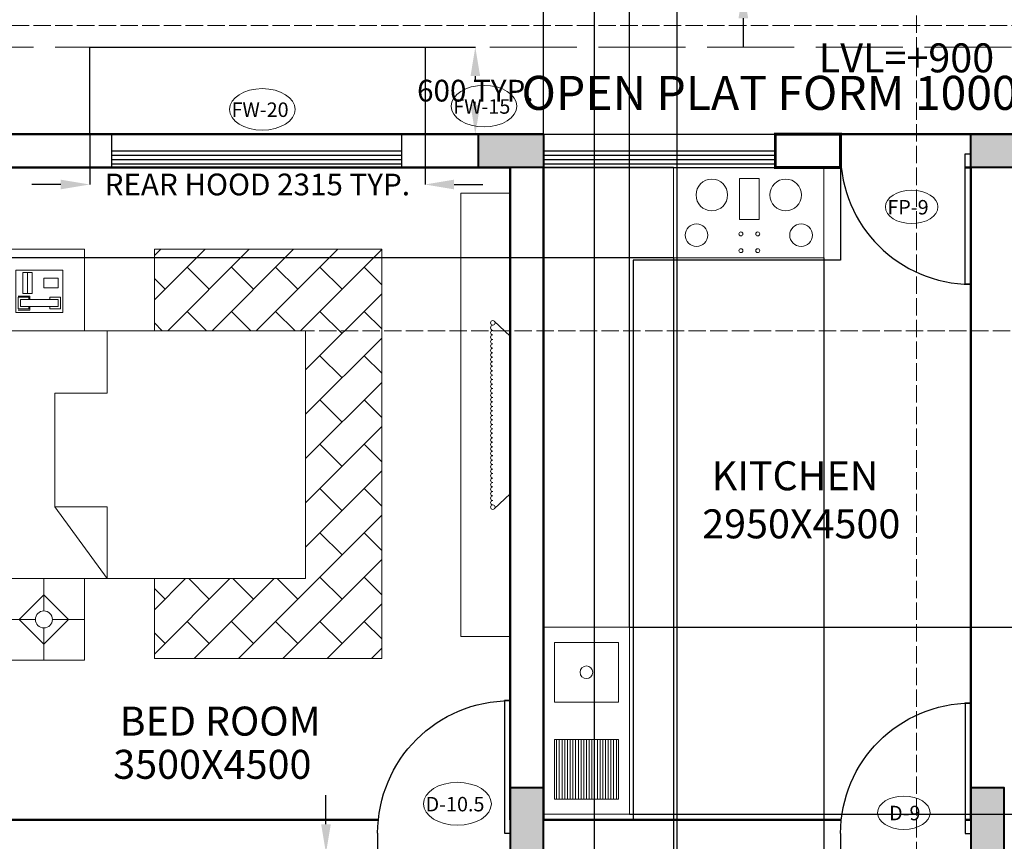
# Model space of a CAD drawing. Units: inches. Extents: x 22626 to 57351, y 2118 to 36234.
# Tile 5 of 10: x 34432 to 41227, y 23379 to 29046. Entities that reach past the tile are written whole.
import ezdxf

# ---------------------------------------------------------------- set-up
doc = ezdxf.new("R2010")
doc.units = ezdxf.units.IN
doc.header["$MEASUREMENT"] = 0
doc.linetypes.add('ACAD_ISO02W100', pattern=[15, 12, -3])
for name, color, linetype, lineweight in [('A-ANNO-DIMS', 130, 'Continuous', 18), ('A-ANNO-IDEN', 130, 'Continuous', 15), ('A-ANNO-SYMB', 130, 'Continuous', 18), ('A-AREA-IDEN', 130, 'Continuous', 18), ('A-COLS', 7, 'Continuous', 40), ('A-EQPM', 30, 'Continuous', 18), ('A-FIXT-PATT', 8, 'Continuous', 13), ('A-FLOR-CASE', 30, 'Continuous', 25), ('A-FLOR-FIXT', 30, 'Continuous', 18), ('A-ROOF', 80, 'Continuous', 25), ('A-ROOF-OVHD', 80, 'ACAD_ISO02W100', 18), ('A-WALL', 80, 'Continuous', 50), ('DOORS', 32, 'Continuous', 25), ('FURNITURE', 30, 'Continuous', 18), ('WINDOWS', 212, 'Continuous', 25)]:
    doc.layers.add(name, color=color, linetype=linetype, lineweight=lineweight)
doc.layers.add('A-SECT', color=2, linetype='ACAD_ISO02W100', lineweight=18, true_color=0xf1eb1f)
doc.styles.get("Standard").update_dxf_attribs({"font": 'arial.ttf'})
doc.dimstyles.get("Standard").update_dxf_attribs({"dimtxt": 150, "dimasz": 200, "dimexe": 0.18, "dimexo": 0.0625, "dimgap": 0.09, "dimtad": 0, "dimtih": 1, "dimtoh": 1, "dimdec": 0, "dimzin": 0, "dimdsep": 46, "dimtxsty": 'Standard', "dimcen": 0.09, "dimadec": 0, "dimazin": 0, "dimtfac": 1, "dimtdec": 0, "dimtofl": 0, "dimtmove": 0, "dimatfit": 3, "dimfxl": 1, "dimtolj": 1, "dimtzin": 0, "dimarcsym": 0})

# ---------------------------------------------------------------- blocks, each defined once
blk = doc.blocks.new('*U7')
for p, q in [((0, 0), (0, -6)), ((40, 0), (40, -6))]:
    blk.add_line(p, q)
blk.add_lwpolyline([(0, 0), (0, 40), (1.75, 40), (1.75, 0)], close=True)
blk.add_arc((0, 0), 40, 0, 90)
blk = doc.blocks.new('Phone - Desk')
for p, q in [((-4.5, -5), (-4.5, 5)), ((-4.5, 5), (4.5, 5)), ((-4, 4.5), (-4, 2)), ((-3.75, 4.5), (-3.75, 2.25)), ((-1.25, 4.5), (-3.75, 4.5)), ((-1.25, 2.25), (-1.25, 4.5)), ((-1, 2), (-1, 4.5)), ((4.5, 5), (4.5, -5)), ((-3.75, 2.25), (-3.25, 2.25)), ((-3.25, 4), (-3.25, -4)), ((-3.25, 4), (-1.75, 4)), ((-1.75, -4), (-1.75, 4)), ((-1.75, 2.25), (-1.25, 2.25)), ((4, 3.5), (-0.5, 3.5)), ((-0.5, 3.5), (-0.5, 1.5)), ((-0.5, 2.5), (4, 2.5)), ((4, 1.5), (4, 3.5)), ((-4, 2), (-3.25, 2)), ((-1.75, 2), (-1, 2)), ((-0.5, 1.5), (4, 1.5)), ((2.75, -1), (0.75, -1)), ((0.75, -1), (0.75, -4)), ((2.75, -4), (2.75, -1)), ((-3.75, -2.25), (-3.25, -2.25)), ((-3.75, -4.5), (-3.75, -2.25)), ((-3.25, -4), (-1.75, -4)), ((-1.75, -2.25), (-1.25, -2.25)), ((-1.25, -2.25), (-1.25, -4.5)), ((0.75, -4), (2.75, -4)), ((4.5, -5), (-4.5, -5)), ((-1.25, -4.5), (-3.75, -4.5))]:
    blk.add_line(p, q)
blk = doc.blocks.new('BED')
h = blk.add_hatch()
h.set_pattern_fill('AR-B816', color=256, scale=27, angle=45)
h.paths.add_polyline_path([(36405.4, 26900.7), (36405.4, 25190.7), (35361.4, 25190.7), (35361.4, 24640.2), (36930.7, 24640.2), (36930.7, 25190.7), (36930.7, 27463.4), (36405.4, 27463.4), (35361.4, 27463.4), (35361.4, 26900.7)])
for p, q in [((35361.4, 26900.7), (35361.4, 27463.4)), ((35361.4, 27463.4), (36405.4, 27463.4)), ((36405.4, 27463.4), (36930.7, 27463.4)), ((36930.7, 27463.4), (36930.7, 25190.7)), ((35034.9, 26900.7), (35034.9, 26469.4)), ((34673.2, 25686.3), (34673.2, 26469.4)), ((35034.9, 26469.4), (34673.2, 26469.4)), ((35034.9, 25686.3), (34673.2, 25686.3)), ((34673.2, 25686.3), (35034.9, 25190.7)), ((35034.9, 25190.7), (35034.9, 25686.3)), ((34598.8, 25190.7), (34598.8, 24968.4)), ((35361.4, 24640.2), (35361.4, 25190.7)), ((36930.7, 25190.7), (36930.7, 24640.2)), ((34428.6, 24909.4), (34598.8, 25079.6)), ((34598.8, 25079.6), (34768.9, 24909.4)), ((34317.4, 24909.4), (34539.7, 24909.4)), ((34598.8, 24739.2), (34428.6, 24909.4)), ((34768.9, 24909.4), (34598.8, 24739.2)), ((34657.8, 24909.4), (34880.1, 24909.4)), ((34598.8, 24850.4), (34598.8, 24628.1)), ((36930.7, 24640.2), (35361.4, 24640.2))]:
    blk.add_line(p, q)
for points in [[(34317.4, 26900.7), (34880.1, 26900.7), (34880.1, 27463.4), (34317.4, 27463.4)], [(34317.4, 26900.7), (36405.4, 26900.7), (36405.4, 25190.7), (34317.4, 25190.7)], [(34317.4, 25190.7), (34880.1, 25190.7), (34880.1, 24628.1), (34317.4, 24628.1)]]:
    blk.add_lwpolyline(points, close=True)
blk.add_circle((34598.8, 24909.4), 59)
at = {"xscale": 32.52267765020765, "yscale": 32.52267765020765, "zscale": 32.52267765020765, "rotation": 90}
blk.add_blockref('Phone - Desk', (34567, 27172.9), dxfattribs=at)
blk = doc.blocks.new('*D20')
at = {"layer": 'A-ANNO-DIMS', "color": 0, "lineweight": -2, "transparency": 16777216}
for p, q in [((39426.2, 29756.9), (39426.2, 29956.9)), ((40218, 29556.9), (39426, 29556.9)), ((40218, 29256.9), (39426, 29256.9)), ((39426.2, 29056.9), (39426.2, 28856.9))]:
    blk.add_line(p, q, dxfattribs=at)
at = {"layer": 'A-ANNO-DIMS', "color": 0, "transparency": 16777216}
for points in [[(39392.9, 29756.9), (39459.5, 29756.9), (39426.2, 29556.9)], [(39392.9, 29056.9), (39459.5, 29056.9), (39426.2, 29256.9)]]:
    blk.add_solid(points, dxfattribs=at)
at = {"layer": 'Defpoints', "color": 0, "transparency": 16777216}
for p in [(39426.2, 29556.9), (40218, 29556.9), (40218, 29256.9)]:
    blk.add_point(p, dxfattribs=at)
at = {"layer": 'A-ANNO-DIMS', "color": 0, "transparency": 16777216, "insert": (39426.2, 29406.9), "char_height": 150, "attachment_point": 5}
blk.add_mtext('\\A1;300', dxfattribs=at)
blk = doc.blocks.new('BEDROOM-WALL-UNIT-LARGE')
for p, q in [((340.4, 2073.4), (230, 2176.6)), ((340.4, 2073.4), (340.4, 984.3)), ((340.4, 984.3), (230, 881.1))]:
    blk.add_line(p, q)
blk.add_lwpolyline([(340.4, 3057.7), (0, 3057.7), (0, 0), (340.4, 0)], close=True)
for centre in [(220.4, 2164.5), (220.4, 893.2)]:
    blk.add_circle(centre, 15.4)
for centre, radius, start, end in [((223.5, 2130.6), 18.8, 99.47834, 260.52166), ((220.4, 2096.6), 15.4, 90, 270), ((220.4, 2065.7), 15.4, 90, 270), ((220.4, 2034.9), 15.4, 90, 270), ((220.4, 2004), 15.4, 90, 270), ((220.4, 1973.2), 15.4, 90, 270), ((220.4, 1942.3), 15.4, 90, 270), ((220.4, 1911.5), 15.4, 90, 270), ((220.4, 1880.6), 15.4, 90, 270), ((220.4, 1849.7), 15.4, 90, 270), ((220.4, 1818.9), 15.4, 90, 270), ((220.4, 1788), 15.4, 90, 270), ((220.4, 1757.2), 15.4, 90, 270), ((220.4, 1726.3), 15.4, 90, 270), ((220.4, 1695.5), 15.4, 90, 270), ((220.4, 1664.6), 15.4, 90, 270), ((220.4, 1633.8), 15.4, 90, 270), ((220.4, 1602.9), 15.4, 90, 270), ((220.4, 1572), 15.4, 90, 270), ((220.4, 1541.2), 15.4, 90, 270), ((220.4, 1510.3), 15.4, 90, 270), ((220.4, 1479.5), 15.4, 90, 270), ((220.4, 1448.6), 15.4, 90, 270), ((220.4, 1417.8), 15.4, 90, 270), ((220.4, 1386.9), 15.4, 90, 270), ((220.4, 1356), 15.4, 90, 270), ((220.4, 1325.2), 15.4, 90, 270), ((220.4, 1294.3), 15.4, 90, 270), ((220.4, 1263.5), 15.4, 90, 270), ((220.4, 1232.6), 15.4, 90, 270), ((220.4, 1201.8), 15.4, 90, 270), ((220.4, 1170.9), 15.4, 90, 270), ((220.4, 1140), 15.4, 90, 270), ((220.4, 1109.2), 15.4, 90, 270), ((220.4, 1078.3), 15.4, 90, 270), ((220.4, 1047.5), 15.4, 90, 270), ((220.4, 1016.6), 15.4, 90, 270), ((220.4, 985.8), 15.4, 90, 270), ((220.4, 954.9), 15.4, 90, 270), ((220.4, 924), 15.4, 90, 270)]:
    blk.add_arc(centre, radius, start, end)
blk = doc.blocks.new('WIN-FIXED-2000-REAR')
for p, q in [((0, 114.3), (2000, 114.3)), ((0, 84.3), (2000, 84.3)), ((0, 54.3), (2000, 54.3)), ((0, 24.3), (2000, 24.3))]:
    blk.add_line(p, q)
blk.add_lwpolyline([(0, 230), (2000, 230), (2000, 0), (0, 0), (0, 230)])
blk = doc.blocks.new('COL-RECTANGULAR')
h = blk.add_hatch(color=256)
h.dxf.hatch_style = 1
h.paths.add_polyline_path([(0, 0), (450, 0), (450, 230), (0, 230)])
blk.add_lwpolyline([(0, 0), (0, 230), (450, 230), (450, 0)], close=True)
blk = doc.blocks.new('WINDOW-HOOD')
for p, q in [((0, 0), (0, 600)), ((0, 600), (2314.6, 600)), ((2314.6, 600), (2314.6, 0))]:
    blk.add_line(p, q)
blk = doc.blocks.new('*D53')
at = {"layer": 'A-ANNO-DIMS', "color": 0, "lineweight": -2, "transparency": 16777216}
for p, q in [((36545.6, 23496.9), (36545.6, 23696.9)), ((36412.5, 23296.9), (36545.7, 23296.9)), ((36412.5, 22941.5), (36545.7, 22941.5)), ((36545.6, 22741.5), (36545.6, 22541.5))]:
    blk.add_line(p, q, dxfattribs=at)
at = {"layer": 'A-ANNO-DIMS', "color": 0, "transparency": 16777216}
for points in [[(36512.2, 23496.9), (36578.9, 23496.9), (36545.6, 23296.9)], [(36512.2, 22741.5), (36578.9, 22741.5), (36545.6, 22941.5)]]:
    blk.add_solid(points, dxfattribs=at)
at = {"layer": 'Defpoints', "color": 0, "transparency": 16777216}
for p in [(36412.4, 23296.9), (36545.6, 23296.9), (36412.4, 22941.5)]:
    blk.add_point(p, dxfattribs=at)
at = {"layer": 'A-ANNO-DIMS', "color": 0, "transparency": 16777216, "insert": (36545.6, 23119.2), "char_height": 150, "attachment_point": 5}
blk.add_mtext('\\A1;355 TYP.', dxfattribs=at)
blk = doc.blocks.new('*D86')
at = {"layer": 'A-ANNO-DIMS', "color": 0, "lineweight": -2, "transparency": 16777216}
for p, q in [((34914.8, 28256.8), (34914.8, 27909.5)), ((37229.4, 28256.8), (37229.4, 27909.5)), ((34714.8, 27909.7), (34514.8, 27909.7)), ((37429.4, 27909.7), (37629.4, 27909.7))]:
    blk.add_line(p, q, dxfattribs=at)
at = {"layer": 'A-ANNO-DIMS', "color": 0, "transparency": 16777216}
for points in [[(34714.8, 27943), (34714.8, 27876.3), (34914.8, 27909.7)], [(37429.4, 27943), (37429.4, 27876.3), (37229.4, 27909.7)]]:
    blk.add_solid(points, dxfattribs=at)
at = {"layer": 'Defpoints', "color": 0, "transparency": 16777216}
for p in [(34914.8, 28256.9), (37229.4, 28256.9), (37229.4, 27909.7)]:
    blk.add_point(p, dxfattribs=at)
at = {"layer": 'A-ANNO-DIMS', "color": 0, "transparency": 16777216, "insert": (36072.1, 27909.7), "char_height": 150, "attachment_point": 5}
blk.add_mtext('\\A1;REAR HOOD 2315 TYP.', dxfattribs=at)
blk = doc.blocks.new('*D87')
at = {"layer": 'A-ANNO-DIMS', "color": 0, "lineweight": -2, "transparency": 16777216}
for p, q in [((37229.4, 28856.9), (37576.7, 28856.9)), ((37576.5, 28656.9), (37576.5, 28633.5)), ((37576.5, 28456.9), (37576.5, 28480.2)), ((37229.4, 28256.9), (37576.7, 28256.9))]:
    blk.add_line(p, q, dxfattribs=at)
at = {"layer": 'A-ANNO-DIMS', "color": 0, "transparency": 16777216}
for points in [[(37543.2, 28656.9), (37609.9, 28656.9), (37576.5, 28856.9)], [(37543.2, 28456.9), (37609.9, 28456.9), (37576.5, 28256.9)]]:
    blk.add_solid(points, dxfattribs=at)
at = {"layer": 'Defpoints', "color": 0, "transparency": 16777216}
for p in [(37229.4, 28856.9), (37576.5, 28856.9), (37229.4, 28256.9)]:
    blk.add_point(p, dxfattribs=at)
at = {"layer": 'A-ANNO-DIMS', "color": 0, "transparency": 16777216, "insert": (37576.5, 28556.9), "char_height": 150, "attachment_point": 5}
blk.add_mtext('\\A1;600 TYP.', dxfattribs=at)
blk = doc.blocks.new('*D99')
at = {"layer": 'A-ANNO-DIMS', "color": 0, "lineweight": -2, "transparency": 16777216}
for p, q in [((41184.6, 30456.9), (57038.8, 30456.9)), ((57038.6, 30256.9), (57038.6, 18933.6)), ((57038.6, 7456.9), (57038.6, 18780.1)), ((43702.5, 7256.9), (57038.8, 7256.9))]:
    blk.add_line(p, q, dxfattribs=at)
at = {"layer": 'A-ANNO-DIMS', "color": 0, "transparency": 16777216}
for points in [[(57005.3, 30256.9), (57071.9, 30256.9), (57038.6, 30456.9)], [(57005.3, 7456.9), (57071.9, 7456.9), (57038.6, 7256.9)]]:
    blk.add_solid(points, dxfattribs=at)
at = {"layer": 'Defpoints', "color": 0, "transparency": 16777216}
for p in [(41184.5, 30456.9), (57038.6, 30456.9), (43702.4, 7256.9)]:
    blk.add_point(p, dxfattribs=at)
at = {"layer": 'A-ANNO-DIMS', "color": 0, "transparency": 16777216, "insert": (57038.6, 18856.9), "char_height": 150, "attachment_point": 5}
blk.add_mtext('\\A1;23200', dxfattribs=at)
blk = doc.blocks.new('*D106')
at = {"layer": 'A-ANNO-DIMS', "color": 0, "lineweight": -2, "transparency": 16777216}
for p, q in [((38198.3, 36136.1), (37998.3, 36136.1)), ((38398.3, 21952.1), (38398.3, 36136.2)), ((38968.9, 21952.1), (38968.9, 36136.2)), ((39168.9, 36136.1), (39368.9, 36136.1))]:
    blk.add_line(p, q, dxfattribs=at)
at = {"layer": 'A-ANNO-DIMS', "color": 0, "transparency": 16777216}
for points in [[(38198.3, 36169.4), (38198.3, 36102.7), (38398.3, 36136.1)], [(39168.9, 36169.4), (39168.9, 36102.7), (38968.9, 36136.1)]]:
    blk.add_solid(points, dxfattribs=at)
at = {"layer": 'Defpoints', "color": 0, "transparency": 16777216}
for p in [(38968.9, 36136.1), (38398.3, 21952.1), (38968.9, 21952.1)]:
    blk.add_point(p, dxfattribs=at)
at = {"layer": 'A-ANNO-DIMS', "color": 0, "transparency": 16777216, "insert": (38683.6, 36136.1), "char_height": 150, "attachment_point": 5}
blk.add_mtext('\\A1;570.6', dxfattribs=at)
blk = doc.blocks.new('*D108')
at = {"layer": 'A-ANNO-DIMS', "color": 0, "lineweight": -2, "transparency": 16777216}
for p, q in [((37847.4, 36136.1), (37647.4, 36136.1)), ((38047.4, 24856.2), (38047.4, 36136.2)), ((38641, 24856.2), (38641, 36136.2)), ((38841, 36136.1), (39041, 36136.1))]:
    blk.add_line(p, q, dxfattribs=at)
at = {"layer": 'A-ANNO-DIMS', "color": 0, "transparency": 16777216}
for points in [[(37847.4, 36169.4), (37847.4, 36102.7), (38047.4, 36136.1)], [(38841, 36169.4), (38841, 36102.7), (38641, 36136.1)]]:
    blk.add_solid(points, dxfattribs=at)
at = {"layer": 'Defpoints', "color": 0, "transparency": 16777216}
for p in [(38641, 36136.1), (38047.4, 24856.1), (38641, 24856.1)]:
    blk.add_point(p, dxfattribs=at)
at = {"layer": 'A-ANNO-DIMS', "color": 0, "transparency": 16777216, "insert": (38344.2, 36136.1), "char_height": 150, "attachment_point": 5}
blk.add_mtext('\\A1;593.6', dxfattribs=at)
blk = doc.blocks.new('*D109')
at = {"layer": 'A-ANNO-DIMS', "color": 0, "lineweight": -2, "transparency": 16777216}
for p, q in [((38641.1, 24856.1), (57038.8, 24856.1)), ((57038.6, 24656.1), (57038.6, 24287.5)), ((57038.6, 23765.5), (57038.6, 24134.1)), ((38641.1, 23565.5), (57038.8, 23565.5))]:
    blk.add_line(p, q, dxfattribs=at)
at = {"layer": 'A-ANNO-DIMS', "color": 0, "transparency": 16777216}
for points in [[(57005.3, 24656.1), (57071.9, 24656.1), (57038.6, 24856.1)], [(57005.3, 23765.5), (57071.9, 23765.5), (57038.6, 23565.5)]]:
    blk.add_solid(points, dxfattribs=at)
at = {"layer": 'Defpoints', "color": 0, "transparency": 16777216}
for p in [(38641, 24856.1), (57038.6, 24856.1), (38641, 23565.5)]:
    blk.add_point(p, dxfattribs=at)
at = {"layer": 'A-ANNO-DIMS', "color": 0, "transparency": 16777216, "insert": (57038.6, 24210.8), "char_height": 150, "attachment_point": 5}
blk.add_mtext('\\A1;1290.6', dxfattribs=at)
blk = doc.blocks.new('*D110')
at = {"layer": 'A-ANNO-DIMS', "color": 0, "lineweight": -2, "transparency": 16777216}
for p, q in [((38945.2, 27402.7), (38945.2, 2216.2)), ((39982.4, 27402.7), (39982.4, 2216.2)), ((39145.2, 2216.4), (39160.2, 2216.4)), ((39782.4, 2216.4), (39767.4, 2216.4))]:
    blk.add_line(p, q, dxfattribs=at)
at = {"layer": 'A-ANNO-DIMS', "color": 0, "transparency": 16777216}
for points in [[(39145.2, 2249.7), (39145.2, 2183), (38945.2, 2216.4)], [(39782.4, 2249.7), (39782.4, 2183), (39982.4, 2216.4)]]:
    blk.add_solid(points, dxfattribs=at)
at = {"layer": 'Defpoints', "color": 0, "transparency": 16777216}
for p in [(38945.2, 27402.8), (39982.4, 27402.8), (39982.4, 2216.4)]:
    blk.add_point(p, dxfattribs=at)
at = {"layer": 'A-ANNO-DIMS', "color": 0, "transparency": 16777216, "insert": (39463.8, 2216.4), "char_height": 150, "attachment_point": 5}
blk.add_mtext('\\A1;1037.2', dxfattribs=at)
blk = doc.blocks.new('*D111')
at = {"layer": 'A-ANNO-DIMS', "color": 0, "lineweight": -2, "transparency": 16777216}
for p, q in [((38945.1, 28026.9), (22909.9, 28026.9)), ((22910.1, 27826.9), (22910.1, 27791.5)), ((22910.1, 27602.8), (22910.1, 27638.2)), ((38945.1, 27402.8), (22909.9, 27402.8))]:
    blk.add_line(p, q, dxfattribs=at)
at = {"layer": 'A-ANNO-DIMS', "color": 0, "transparency": 16777216}
for points in [[(22876.7, 27826.9), (22943.4, 27826.9), (22910.1, 28026.9)], [(22876.7, 27602.8), (22943.4, 27602.8), (22910.1, 27402.8)]]:
    blk.add_solid(points, dxfattribs=at)
at = {"layer": 'Defpoints', "color": 0, "transparency": 16777216}
for p in [(22910.1, 28026.9), (38945.2, 28026.9), (38945.2, 27402.8)]:
    blk.add_point(p, dxfattribs=at)
at = {"layer": 'A-ANNO-DIMS', "color": 0, "transparency": 16777216, "insert": (22910.1, 27714.8), "char_height": 150, "attachment_point": 5}
blk.add_mtext('\\A1;624', dxfattribs=at)

msp = doc.modelspace()

# ---------------------------------------------------------------- hatches: boundary and pattern name
at = {"layer": 'A-FIXT-PATT'}
h = msp.add_hatch(dxfattribs=at)
h.set_pattern_fill('ANSI31', color=256, scale=150, angle=45)
h.paths.add_polyline_path([(38564.3, 24082.24), (38122.86, 24082.24), (38122.86, 23670.51), (38564.3, 23670.51)])

# ---------------------------------------------------------------- linework, layer by layer
at = {"layer": 'A-ANNO-IDEN'}
for centre, major_axis in [((36106.3, 28427.77), (226.15, 0)), ((37636.64, 28450.02), (226.15, 0)), ((40588.03, 27754.96), (181.33, 0)), ((37453.29, 23637.49), (233.77, 0)), ((40533.83, 23576.08), (181.33, 0))]:
    msp.add_ellipse(centre, major_axis=major_axis, ratio=0.634255, start_param=-1.5707963, end_param=4.712389, dxfattribs=at)
at = {"layer": 'A-EQPM'}
for p, q in [((38945.2, 27402.81), (38945.2, 28026.86)), ((39982.43, 27402.81), (39982.43, 28026.86)), ((39982.43, 27402.81), (38945.2, 27402.81))]:
    msp.add_line(p, q, dxfattribs=at)
msp.add_lwpolyline([(39400.74, 27951.13), (39534.54, 27951.13), (39534.54, 27667.46), (39400.74, 27667.46)], close=True, dxfattribs=at)
for centre, radius in [((39208.84, 27837.93), 109.16), ((39718.79, 27837.93), 109.16), ((39102.98, 27559.64), 77.98), ((39824.64, 27559.64), 77.98), ((39409.65, 27568.67), 13.61), ((39525.63, 27568.67), 13.61), ((39409.65, 27453.11), 13.61), ((39525.63, 27453.11), 13.61)]:
    msp.add_circle(centre, radius, dxfattribs=at)
at = {"layer": 'A-FLOR-CASE'}
for p, q in [((40097.43, 28026.86), (40097.43, 27387.39)), ((40097.43, 27387.39), (38665.05, 27387.39)), ((38665.05, 27387.39), (38665.05, 23526.86))]:
    msp.add_line(p, q, dxfattribs=at)
at = {"layer": 'A-FLOR-FIXT'}
for p, q in [((38047.43, 24856.11), (38665.05, 24856.11)), ((38641.03, 24856.11), (38641.03, 23565.5)), ((38047.43, 23565.5), (38641.03, 23565.5))]:
    msp.add_line(p, q, dxfattribs=at)
for points in [[(38122.86, 24339.37), (38564.3, 24339.37), (38564.3, 24751.09), (38122.86, 24751.09)], [(38122.86, 24082.24), (38564.3, 24082.24), (38564.3, 23670.51), (38122.86, 23670.51)]]:
    msp.add_lwpolyline(points, close=True, dxfattribs=at)
msp.add_circle((38343.58, 24545.23), 43.7, dxfattribs=at)
at = {"layer": 'A-ROOF-OVHD', "ltscale": 10}
msp.add_lwpolyline([(33177.24, 29006.86), (33177.24, 29006.86), (48950.76, 29006.86), (48950.76, 28256.86)], dxfattribs=at)
at = {"layer": 'A-ROOF-OVHD', "ltscale": 50}
msp.add_lwpolyline([(33177.24, 28256.86), (33177.24, 28856.86), (48007.84, 28856.86), (48007.84, 28256.86)], dxfattribs=at)
at = {"layer": 'A-SECT', "ltscale": 10}
for p, q in [((40622.43, 34176.08), (40622.43, 4176.35)), ((55067.61, 26900.74), (24870.06, 26900.74))]:
    msp.add_line(p, q, dxfattribs=at)
at = {"layer": 'A-WALL'}
for p, q in [((34087.43, 28256.86), (38047.43, 28256.86)), ((40097.43, 28256.86), (42842.43, 28256.86)), ((40997.43, 28256.86), (41447.43, 28256.86)), ((34317.43, 28026.86), (37817.43, 28026.86)), ((37817.43, 28026.86), (37817.43, 23526.86)), ((38047.43, 28026.86), (38047.43, 23526.86)), ((40958.05, 28026.86), (40997.43, 28026.86)), ((40997.43, 28026.86), (40997.43, 23526.86)), ((36907.14, 23526.86), (34317.43, 23526.86)), ((40102.46, 23526.86), (38047.43, 23526.86)), ((40997.43, 23526.86), (40958.05, 23526.86))]:
    msp.add_line(p, q, dxfattribs=at)
at = {"layer": 'A-WALL', "const_width": 20}
msp.add_lwpolyline([(39647.43, 28026.86), (39647.43, 28256.86), (40097.43, 28256.86), (40097.43, 28026.86)], close=True, dxfattribs=at)
at = {"layer": 'WINDOWS'}
for p, q in [((38047.43, 28256.86), (39647.43, 28256.86)), ((38047.43, 28141.36), (39647.43, 28141.36)), ((38047.43, 28111.36), (39647.43, 28111.36)), ((38047.43, 28081.36), (39647.43, 28081.36)), ((38047.43, 28051.36), (39647.43, 28051.36)), ((38047.43, 28026.86), (39647.43, 28026.86))]:
    msp.add_line(p, q, dxfattribs=at)

# ---------------------------------------------------------------- block references
at = {"layer": 'A-COLS'}
for p in [(37597.43, 28026.86), (40997.43, 28026.86)]:
    msp.add_blockref('COL-RECTANGULAR', p, dxfattribs=at)
at = {"layer": 'A-COLS', "extrusion": (0, 0, -1), "zscale": -1, "rotation": 90}
for p in [(-37817.43, 23296.86), (-40997.43, 23296.86)]:
    msp.add_blockref('COL-RECTANGULAR', p, dxfattribs=at)
at = {"layer": 'A-ROOF'}
msp.add_blockref('WINDOW-HOOD', (34914.77, 28256.86), dxfattribs=at)
at = {"layer": 'DOORS', "xscale": 22.5, "yscale": 22.5, "zscale": 22.5, "rotation": 180}
msp.add_blockref('*U7', (40997.43, 28121.86), dxfattribs=at)
at = {"layer": 'DOORS'}
for p, xscale, yscale, zscale in [((37817.43, 23434.11), -22.875, 22.875, 22.875), ((40997.43, 23431.86), -22.5, 22.5, 22.5)]:
    msp.add_blockref('*U7', p, dxfattribs=dict(at, xscale=xscale, yscale=yscale, zscale=zscale))
at = {"layer": 'FURNITURE'}
for name, p in [('BEDROOM-WALL-UNIT-LARGE', (37477.04, 24791.01)), ('BED', (0, 0))]:
    msp.add_blockref(name, p, dxfattribs=at)
at = {"layer": 'WINDOWS'}
msp.add_blockref('WIN-FIXED-2000-REAR', (35067.43, 28026.86), dxfattribs=at)

# ---------------------------------------------------------------- texts
at = {"layer": 'A-ANNO-IDEN'}
for s, p in [('FW-20', (35893.87, 28375.49)), ('FW-15', (37424.2, 28397.74)), ('FP-9', (40420.41, 27702.68)), ('D-10.5', (37233.23, 23585.21)), ('D-9', (40431.99, 23523.8))]:
    msp.add_text(s, height=100, dxfattribs=at).set_placement(p)
at = {"layer": 'A-ANNO-SYMB'}
msp.add_text('LVL=+900', height=200, dxfattribs=at).set_placement((39946.96, 28683.24))
at = {"layer": 'A-AREA-IDEN'}
for s, height, p in [('OPEN PLAT FORM 1000 WIDE', 234.5284, (37895.41, 28424.5)), ('KITCHEN', 200, (39208.02, 25800.4)), ('2950X4500', 200, (39142.09, 25468.71)), ('BED ROOM', 200, (35121.14, 24107.94)), ('3500X4500', 200, (35077.55, 23809.83))]:
    msp.add_text(s, height=height, dxfattribs=at).set_placement(p)

# ---------------------------------------------------------------- dimensions: what is measured, and where the dimension line sits
at = {"layer": 'A-ANNO-DIMS'}
for base, p1, p2, picture, middle in [((38641.03, 36136.06), (38047.43, 24856.11), (38641.03, 24856.11), '*D108', (38344.23, 36136.06)), ((38968.9273, 36136.0593), (38398.2788, 21952.0585), (38968.9273, 21952.0585), '*D106', (38683.603, 36136.0593)), ((39982.43, 2216.37), (38945.2, 27402.81), (39982.43, 27402.81), '*D110', (39463.81, 2216.37))]:
    dim = msp.add_linear_dim(base=base, p1=p1, p2=p2, dimstyle='Standard', override={"dimdec": 1, "dimlfac": 1, "dimrnd": 0, "dimzin": 0, "dimdsep": 46, "dimlunit": 2}, dxfattribs=at)
    dim.commit()
    dim.dimension.update_dxf_attribs({"geometry": picture, "text_midpoint": middle})
for base, p1, p2, override, picture, middle in [((57038.61, 30456.86), (43702.43, 7256.86), (41184.53, 30456.86), {"dimdec": 0, "dimlfac": 1, "dimrnd": 0, "dimzin": 0, "dimdsep": 46, "dimlunit": 2}, '*D99', (57038.61, 18856.86)), ((22910.07, 28026.86), (38945.2, 27402.81), (38945.2, 28026.86), {"dimdec": 0, "dimlfac": 1, "dimrnd": 0, "dimzin": 0, "dimdsep": 46, "dimlunit": 2}, '*D111', (22910.07, 27714.84)), ((57038.61, 24856.11), (38641.03, 23565.5), (38641.03, 24856.11), {"dimdec": 1, "dimlfac": 1, "dimrnd": 0, "dimzin": 0, "dimdsep": 46, "dimlunit": 2}, '*D109', (57038.61, 24210.8))]:
    dim = msp.add_linear_dim(base=base, p1=p1, p2=p2, angle=90, dimstyle='Standard', override=override, dxfattribs=at)
    dim.commit()
    dim.dimension.update_dxf_attribs({"geometry": picture, "text_midpoint": middle})
dim = msp.add_linear_dim(base=(39426.18, 29556.86), p1=(40218.02, 29256.86), p2=(40218.02, 29556.86), angle=90, dimstyle='Standard', override={"dimclrd": 0, "dimclre": 0, "dimclrt": 0}, dxfattribs=at)
dim.commit()
dim.dimension.update_dxf_attribs({"geometry": '*D20', "text_midpoint": (39426.18, 29406.86), "dimtype": 160})
for base, p1, p2, picture, middle in [((37576.55, 28856.86), (37229.36, 28256.86), (37229.36, 28856.86), '*D87', (37576.55, 28556.86)), ((36545.55, 23296.86), (36412.43, 22941.54), (36412.43, 23296.86), '*D53', (36545.55, 23119.2))]:
    dim = msp.add_linear_dim(base=base, p1=p1, p2=p2, angle=90, text='<> TYP.', dimstyle='Standard', override={"dimdec": 0, "dimlfac": 1, "dimrnd": 0, "dimzin": 0, "dimdsep": 46, "dimlunit": 2}, dxfattribs=at)
    dim.commit()
    dim.dimension.update_dxf_attribs({"geometry": picture, "text_midpoint": middle})
dim = msp.add_linear_dim(base=(37229.36, 27909.67), p1=(34914.77, 28256.86), p2=(37229.36, 28256.86), text='REAR HOOD <> TYP.', dimstyle='Standard', override={"dimdec": 0, "dimlfac": 1, "dimrnd": 0, "dimzin": 0, "dimdsep": 46, "dimlunit": 2}, dxfattribs=at)
dim.commit()
dim.dimension.update_dxf_attribs({"geometry": '*D86', "text_midpoint": (36072.06, 27909.67)})

doc.saveas('drawing.dxf')
